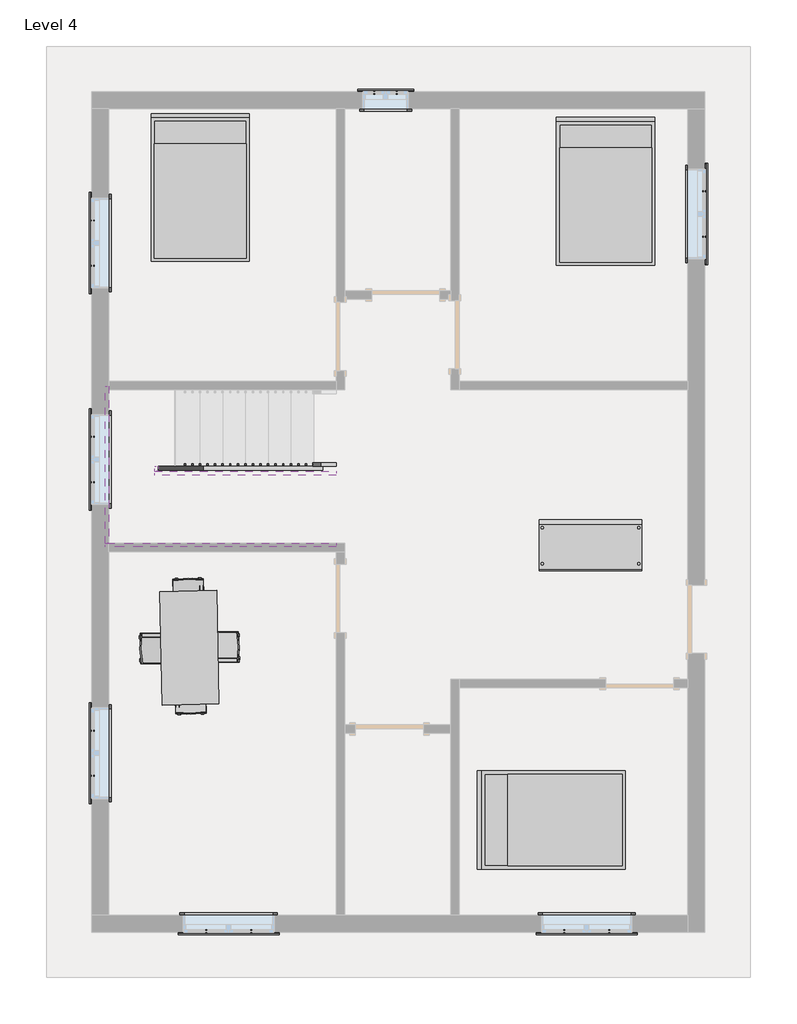
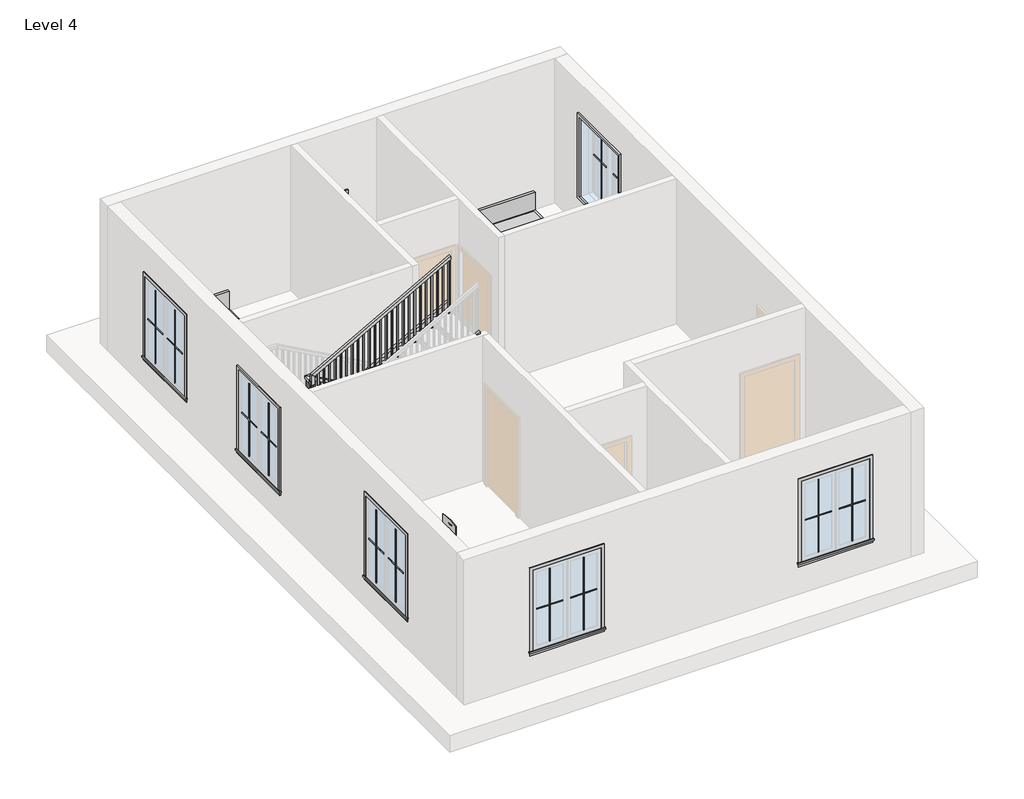
# One storey, part 2 of 2: 29 proxies, 6 members, 4 furniture elements, 1 railing.
"""IFC4 building model written with IfcOpenShell, lengths in millimetres."""

from ifc_helpers import new_model, si_unit, frame, origin, place, context, project, spatial, polyline, outline, extrude, faceted_brep, transform, mapped, element, save
from components import modern_coffee_table_17989_modern_coffee_table_17989_d3a860c8, muntin_pattern_2x2_muntin_pattern_2x2_6dad3731, muntin_pattern_2x2_muntin_pattern_2x2_a30a3345, muntin_pattern_2x2_muntin_pattern_2x2_53152e2c, muntin_pattern_2x2_muntin_pattern_2x2_e8f3e573, trim_window_exterior_flat_with_sill_92b9b949, trim_window_exterior_flat_with_sill_a665a915, trim_window_interior_flat_picture_frame_3bb882cf, trim_window_interior_flat_picture_frame_d485c387, bed_17739_bed_17739_15c61121, dining_table_w_chairs_11374_0cdfc61b

model = new_model("IFC4")

# Units and contexts
model_context = context("Model", 3, world=origin())
ifc_project = project(units=[si_unit("LENGTHUNIT", "METRE", prefix="MILLI")], contexts=[model_context])

# Site, building, storey
site = spatial("IfcSite", under=ifc_project)
building = spatial("IfcBuilding", under=site)
storey = spatial("IfcBuildingStorey", under=building, Name="Level 4", Elevation=9144.0)

# Proxies
placement = place(None, origin())
modern_coffee_table_17989_modern_coffee_table_17989_shape = modern_coffee_table_17989_modern_coffee_table_17989_d3a860c8(model_context)
element("IfcBuildingElementProxy", 1, Name="Modern_Coffee_Table_17989 : Modern_Coffee_Table_17989", ObjectType="Modern_Coffee_Table_17989 : Modern_Coffee_Table_17989", at=placement, inside=storey, context=model_context, shape_type="MappedRepresentation", body=[
    mapped(modern_coffee_table_17989_modern_coffee_table_17989_shape, transform((7937.5, 8234.1992646, 9144.0), x_axis=(1.0, 0.0, 0.0), y_axis=(0.0, 1.0, 0.0), z_axis=(0.0, 0.0, 1.0))),
])
muntin_pattern_2x2_muntin_pattern_2x2_shape = muntin_pattern_2x2_muntin_pattern_2x2_6dad3731(model_context)
element("IfcBuildingElementProxy", 2, Name="Muntin Pattern_2x2 : Muntin Pattern_2x2", ObjectType="Muntin Pattern_2x2 : Muntin Pattern_2x2", at=placement, inside=storey, context=model_context, shape_type="MappedRepresentation", body=[
    mapped(muntin_pattern_2x2_muntin_pattern_2x2_shape, transform((7961.3125, 2701.925, 10128.25), x_axis=(-1.0, 0.0, 0.0), y_axis=(0.0, -1.0, 0.0), z_axis=(0.0, 0.0, 1.0))),
])
element("IfcBuildingElementProxy", 3, Name="Muntin Pattern_2x2 : Muntin Pattern_2x2", ObjectType="Muntin Pattern_2x2 : Muntin Pattern_2x2", at=placement, inside=storey, context=model_context, shape_type="MappedRepresentation", body=[
    mapped(muntin_pattern_2x2_muntin_pattern_2x2_shape, transform((3154.3625, 2701.925, 10128.25), x_axis=(-1.0, 0.0, 0.0), y_axis=(0.0, -1.0, 0.0), z_axis=(0.0, 0.0, 1.0))),
])
element("IfcBuildingElementProxy", 4, Name="Muntin Pattern_2x2 : Muntin Pattern_2x2", ObjectType="Muntin Pattern_2x2 : Muntin Pattern_2x2", at=placement, inside=storey, context=model_context, shape_type="MappedRepresentation", body=[
    mapped(muntin_pattern_2x2_muntin_pattern_2x2_shape, transform((1025.525, 4789.4875, 10128.25), x_axis=(0.0, 1.0, 0.0), y_axis=(-1.0, 0.0, 0.0), z_axis=(0.0, 0.0, 1.0))),
])
element("IfcBuildingElementProxy", 5, Name="Muntin Pattern_2x2 : Muntin Pattern_2x2", ObjectType="Muntin Pattern_2x2 : Muntin Pattern_2x2", at=placement, inside=storey, context=model_context, shape_type="MappedRepresentation", body=[
    mapped(muntin_pattern_2x2_muntin_pattern_2x2_shape, transform((1025.525, 8732.8375, 10128.25), x_axis=(0.0, 1.0, 0.0), y_axis=(-1.0, 0.0, 0.0), z_axis=(0.0, 0.0, 1.0))),
])
element("IfcBuildingElementProxy", 6, Name="Muntin Pattern_2x2 : Muntin Pattern_2x2", ObjectType="Muntin Pattern_2x2 : Muntin Pattern_2x2", at=placement, inside=storey, context=model_context, shape_type="MappedRepresentation", body=[
    mapped(muntin_pattern_2x2_muntin_pattern_2x2_shape, transform((1025.525, 11637.9625, 10128.25), x_axis=(0.0, 1.0, 0.0), y_axis=(-1.0, 0.0, 0.0), z_axis=(0.0, 0.0, 1.0))),
])
element("IfcBuildingElementProxy", 7, Name="Muntin Pattern_2x2 : Muntin Pattern_2x2", ObjectType="Muntin Pattern_2x2 : Muntin Pattern_2x2", at=placement, inside=storey, context=model_context, shape_type="MappedRepresentation", body=[
    mapped(muntin_pattern_2x2_muntin_pattern_2x2_shape, transform((9236.075, 12634.9125, 10128.25), x_axis=(0.0, -1.0, 0.0), y_axis=(1.0, 0.0, 0.0), z_axis=(0.0, 0.0, 1.0))),
])
muntin_pattern_2x2_muntin_pattern_2x2_2_shape = muntin_pattern_2x2_muntin_pattern_2x2_a30a3345(model_context)
element("IfcBuildingElementProxy", 8, Name="Muntin Pattern_2x2 : Muntin Pattern_2x2", ObjectType="Muntin Pattern_2x2 : Muntin Pattern_2x2", at=placement, inside=storey, context=model_context, shape_type="MappedRepresentation", body=[
    mapped(muntin_pattern_2x2_muntin_pattern_2x2_2_shape, transform((7354.8875, 2701.925, 10128.25), x_axis=(1.0, 0.0, 0.0), y_axis=(0.0, 1.0, 0.0), z_axis=(0.0, 0.0, 1.0))),
])
element("IfcBuildingElementProxy", 9, Name="Muntin Pattern_2x2 : Muntin Pattern_2x2", ObjectType="Muntin Pattern_2x2 : Muntin Pattern_2x2", at=placement, inside=storey, context=model_context, shape_type="MappedRepresentation", body=[
    mapped(muntin_pattern_2x2_muntin_pattern_2x2_2_shape, transform((2547.9375, 2701.925, 10128.25), x_axis=(1.0, 0.0, 0.0), y_axis=(0.0, 1.0, 0.0), z_axis=(0.0, 0.0, 1.0))),
])
element("IfcBuildingElementProxy", 10, Name="Muntin Pattern_2x2 : Muntin Pattern_2x2", ObjectType="Muntin Pattern_2x2 : Muntin Pattern_2x2", at=placement, inside=storey, context=model_context, shape_type="MappedRepresentation", body=[
    mapped(muntin_pattern_2x2_muntin_pattern_2x2_2_shape, transform((1025.525, 5395.9125, 10128.25), x_axis=(0.0, -1.0, 0.0), y_axis=(1.0, 0.0, 0.0), z_axis=(0.0, 0.0, 1.0))),
])
element("IfcBuildingElementProxy", 11, Name="Muntin Pattern_2x2 : Muntin Pattern_2x2", ObjectType="Muntin Pattern_2x2 : Muntin Pattern_2x2", at=placement, inside=storey, context=model_context, shape_type="MappedRepresentation", body=[
    mapped(muntin_pattern_2x2_muntin_pattern_2x2_2_shape, transform((1025.525, 9339.2625, 10128.25), x_axis=(0.0, -1.0, 0.0), y_axis=(1.0, 0.0, 0.0), z_axis=(0.0, 0.0, 1.0))),
])
element("IfcBuildingElementProxy", 12, Name="Muntin Pattern_2x2 : Muntin Pattern_2x2", ObjectType="Muntin Pattern_2x2 : Muntin Pattern_2x2", at=placement, inside=storey, context=model_context, shape_type="MappedRepresentation", body=[
    mapped(muntin_pattern_2x2_muntin_pattern_2x2_2_shape, transform((1025.525, 12244.3875, 10128.25), x_axis=(0.0, -1.0, 0.0), y_axis=(1.0, 0.0, 0.0), z_axis=(0.0, 0.0, 1.0))),
])
element("IfcBuildingElementProxy", 13, Name="Muntin Pattern_2x2 : Muntin Pattern_2x2", ObjectType="Muntin Pattern_2x2 : Muntin Pattern_2x2", at=placement, inside=storey, context=model_context, shape_type="MappedRepresentation", body=[
    mapped(muntin_pattern_2x2_muntin_pattern_2x2_2_shape, transform((9236.075, 12028.4875, 10128.25), x_axis=(0.0, 1.0, 0.0), y_axis=(-1.0, 0.0, 0.0), z_axis=(0.0, 0.0, 1.0))),
])
muntin_pattern_2x2_muntin_pattern_2x2_3_shape = muntin_pattern_2x2_muntin_pattern_2x2_53152e2c(model_context)
element("IfcBuildingElementProxy", 14, Name="Muntin Pattern_2x2 : Muntin Pattern_2x2", ObjectType="Muntin Pattern_2x2 : Muntin Pattern_2x2", at=placement, inside=storey, context=model_context, shape_type="MappedRepresentation", body=[
    mapped(muntin_pattern_2x2_muntin_pattern_2x2_3_shape, transform((4808.5375, 13960.475, 10128.25), x_axis=(1.0, 0.0, 0.0), y_axis=(0.0, 1.0, 0.0), z_axis=(0.0, 0.0, 1.0))),
])
muntin_pattern_2x2_muntin_pattern_2x2_4_shape = muntin_pattern_2x2_muntin_pattern_2x2_e8f3e573(model_context)
element("IfcBuildingElementProxy", 15, Name="Muntin Pattern_2x2 : Muntin Pattern_2x2", ObjectType="Muntin Pattern_2x2 : Muntin Pattern_2x2", at=placement, inside=storey, context=model_context, shape_type="MappedRepresentation", body=[
    mapped(muntin_pattern_2x2_muntin_pattern_2x2_4_shape, transform((5110.1625, 13960.475, 10128.25), x_axis=(-1.0, 0.0, 0.0), y_axis=(0.0, -1.0, 0.0), z_axis=(0.0, 0.0, 1.0))),
])
trim_window_exterior_flat_with_sill_shape = trim_window_exterior_flat_with_sill_92b9b949(model_context)
element("IfcBuildingElementProxy", 16, Name="Trim-Window-Exterior-Flat : with Sill", ObjectType="Trim-Window-Exterior-Flat : with Sill", at=placement, inside=storey, context=model_context, shape_type="MappedRepresentation", body=[
    mapped(trim_window_exterior_flat_with_sill_shape, transform((7658.1, 2692.4, 11582.4), x_axis=(1.0, 0.0, 0.0), y_axis=(0.0, 0.0, 1.0), z_axis=(0.0, -1.0, 0.0))),
])
element("IfcBuildingElementProxy", 17, Name="Trim-Window-Exterior-Flat : with Sill", ObjectType="Trim-Window-Exterior-Flat : with Sill", at=placement, inside=storey, context=model_context, shape_type="MappedRepresentation", body=[
    mapped(trim_window_exterior_flat_with_sill_shape, transform((2851.15, 2692.4, 11582.4), x_axis=(1.0, 0.0, 0.0), y_axis=(0.0, 0.0, 1.0), z_axis=(0.0, -1.0, 0.0))),
])
element("IfcBuildingElementProxy", 18, Name="Trim-Window-Exterior-Flat : with Sill", ObjectType="Trim-Window-Exterior-Flat : with Sill", at=placement, inside=storey, context=model_context, shape_type="MappedRepresentation", body=[
    mapped(trim_window_exterior_flat_with_sill_shape, transform((1016.0, 5092.7, 11582.4), x_axis=(0.0, -1.0, 0.0), y_axis=(0.0, 0.0, 1.0), z_axis=(-1.0, 0.0, 0.0))),
])
element("IfcBuildingElementProxy", 19, Name="Trim-Window-Exterior-Flat : with Sill", ObjectType="Trim-Window-Exterior-Flat : with Sill", at=placement, inside=storey, context=model_context, shape_type="MappedRepresentation", body=[
    mapped(trim_window_exterior_flat_with_sill_shape, transform((1016.0, 9036.05, 11582.4), x_axis=(0.0, -1.0, 0.0), y_axis=(0.0, 0.0, 1.0), z_axis=(-1.0, 0.0, 0.0))),
])
element("IfcBuildingElementProxy", 20, Name="Trim-Window-Exterior-Flat : with Sill", ObjectType="Trim-Window-Exterior-Flat : with Sill", at=placement, inside=storey, context=model_context, shape_type="MappedRepresentation", body=[
    mapped(trim_window_exterior_flat_with_sill_shape, transform((1016.0, 11941.175, 11582.4), x_axis=(0.0, -1.0, 0.0), y_axis=(0.0, 0.0, 1.0), z_axis=(-1.0, 0.0, 0.0))),
])
element("IfcBuildingElementProxy", 21, Name="Trim-Window-Exterior-Flat : with Sill", ObjectType="Trim-Window-Exterior-Flat : with Sill", at=placement, inside=storey, context=model_context, shape_type="MappedRepresentation", body=[
    mapped(trim_window_exterior_flat_with_sill_shape, transform((9245.6, 12331.7, 11582.4), x_axis=(0.0, 1.0, 0.0), y_axis=(0.0, 0.0, 1.0), z_axis=(1.0, 0.0, 0.0))),
])
trim_window_exterior_flat_with_sill_2_shape = trim_window_exterior_flat_with_sill_a665a915(model_context)
element("IfcBuildingElementProxy", 22, Name="Trim-Window-Exterior-Flat : with Sill", ObjectType="Trim-Window-Exterior-Flat : with Sill", at=placement, inside=storey, context=model_context, shape_type="MappedRepresentation", body=[
    mapped(trim_window_exterior_flat_with_sill_2_shape, transform((4959.35, 13970.0, 10972.8), x_axis=(-1.0, 0.0, 0.0), y_axis=(0.0, 0.0, 1.0), z_axis=(0.0, 1.0, 0.0))),
])
trim_window_interior_flat_picture_frame_shape = trim_window_interior_flat_picture_frame_3bb882cf(model_context)
element("IfcBuildingElementProxy", 23, Name="Trim-Window-Interior-Flat : Picture Frame", ObjectType="Trim-Window-Interior-Flat : Picture Frame", at=placement, inside=storey, context=model_context, shape_type="MappedRepresentation", body=[
    mapped(trim_window_interior_flat_picture_frame_shape, transform((7658.1, 2921.0, 11582.4), x_axis=(-1.0, 0.0, 0.0), y_axis=(0.0, 0.0, 1.0), z_axis=(0.0, 1.0, 0.0))),
])
element("IfcBuildingElementProxy", 24, Name="Trim-Window-Interior-Flat : Picture Frame", ObjectType="Trim-Window-Interior-Flat : Picture Frame", at=placement, inside=storey, context=model_context, shape_type="MappedRepresentation", body=[
    mapped(trim_window_interior_flat_picture_frame_shape, transform((2851.15, 2921.0, 11582.4), x_axis=(-1.0, 0.0, 0.0), y_axis=(0.0, 0.0, 1.0), z_axis=(0.0, 1.0, 0.0))),
])
element("IfcBuildingElementProxy", 25, Name="Trim-Window-Interior-Flat : Picture Frame", ObjectType="Trim-Window-Interior-Flat : Picture Frame", at=placement, inside=storey, context=model_context, shape_type="MappedRepresentation", body=[
    mapped(trim_window_interior_flat_picture_frame_shape, transform((1244.6, 5092.7, 11582.4), x_axis=(0.0, 1.0, 0.0), y_axis=(0.0, 0.0, 1.0), z_axis=(1.0, 0.0, 0.0))),
])
element("IfcBuildingElementProxy", 26, Name="Trim-Window-Interior-Flat : Picture Frame", ObjectType="Trim-Window-Interior-Flat : Picture Frame", at=placement, inside=storey, context=model_context, shape_type="MappedRepresentation", body=[
    mapped(trim_window_interior_flat_picture_frame_shape, transform((1244.6, 9036.05, 11582.4), x_axis=(0.0, 1.0, 0.0), y_axis=(0.0, 0.0, 1.0), z_axis=(1.0, 0.0, 0.0))),
])
element("IfcBuildingElementProxy", 27, Name="Trim-Window-Interior-Flat : Picture Frame", ObjectType="Trim-Window-Interior-Flat : Picture Frame", at=placement, inside=storey, context=model_context, shape_type="MappedRepresentation", body=[
    mapped(trim_window_interior_flat_picture_frame_shape, transform((1244.6, 11941.175, 11582.4), x_axis=(0.0, 1.0, 0.0), y_axis=(0.0, 0.0, 1.0), z_axis=(1.0, 0.0, 0.0))),
])
element("IfcBuildingElementProxy", 28, Name="Trim-Window-Interior-Flat : Picture Frame", ObjectType="Trim-Window-Interior-Flat : Picture Frame", at=placement, inside=storey, context=model_context, shape_type="MappedRepresentation", body=[
    mapped(trim_window_interior_flat_picture_frame_shape, transform((9017.0, 12331.7, 11582.4), x_axis=(0.0, -1.0, 0.0), y_axis=(0.0, 0.0, 1.0), z_axis=(-1.0, 0.0, 0.0))),
])
trim_window_interior_flat_picture_frame_2_shape = trim_window_interior_flat_picture_frame_d485c387(model_context)
element("IfcBuildingElementProxy", 29, Name="Trim-Window-Interior-Flat : Picture Frame", ObjectType="Trim-Window-Interior-Flat : Picture Frame", at=placement, inside=storey, context=model_context, shape_type="MappedRepresentation", body=[
    mapped(trim_window_interior_flat_picture_frame_2_shape, transform((4959.35, 13741.4, 10972.8), x_axis=(1.0, 0.0, 0.0), y_axis=(0.0, 0.0, 1.0), z_axis=(0.0, -1.0, 0.0))),
])

# Furniture
bed_17739_bed_17739_shape = bed_17739_bed_17739_15c61121(model_context)
element("IfcFurniture", 30, ObjectType="Bed_17739 : Bed_17739", at=placement, inside=storey, context=model_context, shape_type="MappedRepresentation", body=[
    mapped(bed_17739_bed_17739_shape, transform((2470.15, 12661.9, 9144.0), x_axis=(1.0, 0.0, 0.0), y_axis=(0.0, 1.0, 0.0), z_axis=(0.0, 0.0, 1.0))),
])
element("IfcFurniture", 31, ObjectType="Bed_17739 : Bed_17739", at=placement, inside=storey, context=model_context, shape_type="MappedRepresentation", body=[
    mapped(bed_17739_bed_17739_shape, transform((7912.1, 12611.1, 9144.0), x_axis=(1.0, 0.0, 0.0), y_axis=(0.0, 1.0, 0.0), z_axis=(0.0, 0.0, 1.0))),
])
element("IfcFurniture", 32, ObjectType="Bed_17739 : Bed_17739", at=placement, inside=storey, context=model_context, shape_type="MappedRepresentation", body=[
    mapped(bed_17739_bed_17739_shape, transform((7207.25, 4197.35, 9144.0), x_axis=(0.0, 1.0, 0.0), y_axis=(-1.0, 0.0, 0.0), z_axis=(0.0, 0.0, 1.0))),
])
dining_table_w_chairs_11374_shape = dining_table_w_chairs_11374_0cdfc61b(model_context)
element("IfcFurniture", 33, ObjectType="Dining_Table_w_Chairs_11374", at=placement, inside=storey, context=model_context, shape_type="MappedRepresentation", body=[
    mapped(dining_table_w_chairs_11374_shape, transform((2420.6366388, 6492.5326572, 9144.0), x_axis=(-0.019560245774115807, 0.9998086800909743, 0.0), y_axis=(-0.9998086800909743, -0.019560245774115807, 0.0), z_axis=(0.0, 0.0, 1.0))),
])

# Members
element("IfcMember", 34, ObjectType="Stringer - 2\" Width", at=placement, inside=storey, context=model_context, shape_type="SweptSolid", body=[
    extrude(outline(polyline([(9144.0, 4295.1355783), (9351.5983948, 4295.1355783), (10678.0428392, 1907.5355783), (10329.3641651, 1907.5355783), (9144.0, 4041.1910755), (9144.0, 4295.1355783)])), frame((0.0, 8893.8068332, 0.0), z_axis=(0.0, 1.0, 0.0), x_axis=(0.0, 0.0, 1.0)), (0.0, 0.0, 1.0), 50.8),
])
element("IfcMember", 35, ObjectType="Stringer - 2\" Width", at=placement, inside=storey, context=model_context, shape_type="SweptSolid", body=[
    extrude(outline(polyline([(1856.7355783, 8944.6068332), (1907.5355783, 8944.6068332), (1907.5355783, 8877.3), (1856.7355783, 8877.3), (1856.7355783, 8944.6068332)])), frame((0.0, 0.0, 10439.4), z_axis=(0.0, 0.0, 1.0), x_axis=(1.0, 0.0, 0.0)), (0.0, 0.0, 1.0), 304.8),
])
element("IfcMember", 36, ObjectType="Stringer - 2\" Width", at=placement, inside=storey, context=model_context, shape_type="SweptSolid", body=[
    extrude(outline(polyline([(10875.5983948, 1856.7355783), (10526.9197207, 1856.7355783), (11881.5863873, 4295.1355783), (12230.2650614, 4295.1355783), (10875.5983948, 1856.7355783)])), frame((0.0, 8826.5, 0.0), z_axis=(0.0, 1.0, 0.0), x_axis=(0.0, 0.0, 1.0)), (0.0, 0.0, 1.0), 50.8),
])
element("IfcMember", 37, ObjectType="Stringer - 2\" Width", at=placement, inside=storey, context=model_context, shape_type="SweptSolid", body=[
    extrude(outline(polyline([(9144.0, 4295.1355783), (9351.5983948, 4295.1355783), (10744.2, 1788.4526889), (10744.2, 1244.6), (10697.6617086, 1244.6), (9144.0, 4041.1910755), (9144.0, 4295.1355783)])), frame((0.0, 9969.5, 0.0), z_axis=(0.0, 1.0, 0.0), x_axis=(0.0, 0.0, 1.0)), (0.0, 0.0, 1.0), 50.8),
])
element("IfcMember", 38, ObjectType="Stringer - 2\" Width", at=placement, inside=storey, context=model_context, shape_type="SweptSolid", body=[
    extrude(outline(polyline([(1193.8, 10020.3), (1244.6, 10020.3), (1244.6, 7912.1), (1193.8, 7912.1), (1193.8, 10020.3)])), frame((0.0, 0.0, 10439.4), z_axis=(0.0, 0.0, 1.0), x_axis=(1.0, 0.0, 0.0)), (0.0, 0.0, 1.0), 304.8),
])
element("IfcMember", 39, ObjectType="Stringer - 2\" Width", at=placement, inside=storey, context=model_context, shape_type="SweptSolid", body=[
    extrude(outline(polyline([(10507.3008513, 1193.8), (10439.4, 1193.8), (10439.4, 1699.2000811), (11881.5863873, 4295.1355783), (12230.2650614, 4295.1355783), (10507.3008513, 1193.8)])), frame((0.0, 7861.3, 0.0), z_axis=(0.0, 1.0, 0.0), x_axis=(0.0, 0.0, 1.0)), (0.0, 0.0, 1.0), 50.8),
])

# Railing
element("IfcRailing", 40, ObjectType="Handrail - Rectangular", at=placement, inside=storey, context=model_context, shape_type="SolidModel", body=[
    faceted_brep([(4295.1355783, 8944.6068332, 10227.7333333), (4295.1355783, 8944.6068332, 10169.620221), (4295.1355783, 8995.4068332, 10169.620221), (4295.1355783, 8995.4068332, 10227.7333333), (1932.9355783, 8944.6068332, 11540.0666667), (1882.1355783, 8944.6068332, 11510.1757765), (1882.1355783, 8995.4068332, 11510.1757765), (1932.9355783, 8995.4068332, 11540.0666667), (1932.9355783, 8944.6068332, 11582.4), (1882.1355783, 8944.6068332, 11531.6), (1882.1355783, 8995.4068332, 11531.6), (1932.9355783, 8995.4068332, 11582.4), (1856.7355783, 8944.6068332, 11582.4), (1856.7355783, 8944.6068332, 11531.6), (1805.9355783, 8995.4068332, 11531.6), (1805.9355783, 8995.4068332, 11582.4), (1856.7355783, 8868.4068332, 11582.4), (1856.7355783, 8868.4068332, 11531.6), (1805.9355783, 8868.4068332, 11531.6), (1805.9355783, 8868.4068332, 11582.4), (1856.7355783, 8826.5, 11582.4), (1805.9355783, 8826.5, 11582.4), (1805.9355783, 8775.7, 11531.6), (1856.7355783, 8775.7, 11531.6)], [[[0, 1, 2, 3]], [[1, 0, 4, 5]], [[2, 1, 5, 6]], [[3, 2, 6, 7]], [[0, 3, 7, 4]], [[5, 4, 8, 9]], [[6, 5, 9, 10]], [[7, 6, 10, 11]], [[4, 7, 11, 8]], [[9, 8, 12, 13]], [[10, 9, 13, 14]], [[11, 10, 14, 15]], [[8, 11, 15, 12]], [[13, 12, 16, 17]], [[14, 13, 17, 18]], [[15, 14, 18, 19]], [[12, 15, 19, 16]], [[20, 21, 22, 23]], [[17, 16, 20, 23]], [[18, 17, 23, 22]], [[19, 18, 22, 21]], [[16, 19, 21, 20]]]),
    faceted_brep([(1856.7355783, 8826.5, 11582.4), (1856.7355783, 8775.7, 11531.6), (1805.9355783, 8775.7, 11531.6), (1805.9355783, 8826.5, 11582.4), (1856.7355783, 8826.5, 11693.620221), (1805.9355783, 8826.5, 11723.5111111), (1805.9355783, 8775.7, 11723.5111111), (1856.7355783, 8775.7, 11693.620221)], [[[0, 1, 2, 3]], [[4, 5, 6, 7]], [[1, 0, 4, 7]], [[2, 1, 7, 6]], [[3, 2, 6, 5]], [[0, 3, 5, 4]]]),
    faceted_brep([(1805.9355783, 8826.5, 11723.5111111), (1856.7355783, 8826.5, 11693.620221), (1856.7355783, 8775.7, 11693.620221), (1805.9355783, 8775.7, 11723.5111111), (4295.1355783, 8826.5, 13106.4), (4295.1355783, 8775.7, 13106.4), (4295.1355783, 8775.7, 13048.2868876), (4295.1355783, 8826.5, 13048.2868876)], [[[0, 1, 2, 3]], [[4, 5, 6, 7]], [[1, 0, 4, 7]], [[2, 1, 7, 6]], [[3, 2, 6, 5]], [[0, 3, 5, 4]]]),
    extrude(outline(polyline([(13028.8841099, 4260.2105783), (12022.6666667, 4260.2105783), (12022.6666667, 4279.2605783), (13039.4674432, 4279.2605783), (13028.8841099, 4260.2105783)])), frame((0.0, 8791.575, 0.0), z_axis=(0.0, 1.0, 0.0), x_axis=(0.0, 0.0, 1.0)), (0.0, 0.0, 1.0), 19.05),
    extrude(outline(polyline([(12972.4396654, 4158.6105783), (12022.6666667, 4158.6105783), (12022.6666667, 4177.6605783), (12983.0229988, 4177.6605783), (12972.4396654, 4158.6105783)])), frame((0.0, 8791.575, 0.0), z_axis=(0.0, 1.0, 0.0), x_axis=(0.0, 0.0, 1.0)), (0.0, 0.0, 1.0), 19.05),
    extrude(outline(polyline([(12915.995221, 4057.0105783), (12022.6666667, 4057.0105783), (12022.6666667, 4076.0605783), (12926.5785543, 4076.0605783), (12915.995221, 4057.0105783)])), frame((0.0, 8791.575, 0.0), z_axis=(0.0, 1.0, 0.0), x_axis=(0.0, 0.0, 1.0)), (0.0, 0.0, 1.0), 19.05),
    extrude(outline(polyline([(12859.5507765, 3955.4105783), (11853.3333333, 3955.4105783), (11853.3333333, 3974.4605783), (12870.1341099, 3974.4605783), (12859.5507765, 3955.4105783)])), frame((0.0, 8791.575, 0.0), z_axis=(0.0, 1.0, 0.0), x_axis=(0.0, 0.0, 1.0)), (0.0, 0.0, 1.0), 19.05),
    extrude(outline(polyline([(12803.1063321, 3853.8105783), (11853.3333333, 3853.8105783), (11853.3333333, 3872.8605783), (12813.6896654, 3872.8605783), (12803.1063321, 3853.8105783)])), frame((0.0, 8791.575, 0.0), z_axis=(0.0, 1.0, 0.0), x_axis=(0.0, 0.0, 1.0)), (0.0, 0.0, 1.0), 19.05),
    extrude(outline(polyline([(12746.6618876, 3752.2105783), (11853.3333333, 3752.2105783), (11853.3333333, 3771.2605783), (12757.245221, 3771.2605783), (12746.6618876, 3752.2105783)])), frame((0.0, 8791.575, 0.0), z_axis=(0.0, 1.0, 0.0), x_axis=(0.0, 0.0, 1.0)), (0.0, 0.0, 1.0), 19.05),
    extrude(outline(polyline([(12690.2174432, 3650.6105783), (11684.0, 3650.6105783), (11684.0, 3669.6605783), (12700.8007765, 3669.6605783), (12690.2174432, 3650.6105783)])), frame((0.0, 8791.575, 0.0), z_axis=(0.0, 1.0, 0.0), x_axis=(0.0, 0.0, 1.0)), (0.0, 0.0, 1.0), 19.05),
    extrude(outline(polyline([(12633.7729988, 3549.0105783), (11684.0, 3549.0105783), (11684.0, 3568.0605783), (12644.3563321, 3568.0605783), (12633.7729988, 3549.0105783)])), frame((0.0, 8791.575, 0.0), z_axis=(0.0, 1.0, 0.0), x_axis=(0.0, 0.0, 1.0)), (0.0, 0.0, 1.0), 19.05),
    extrude(outline(polyline([(12577.3285543, 3447.4105783), (11684.0, 3447.4105783), (11684.0, 3466.4605783), (12587.9118876, 3466.4605783), (12577.3285543, 3447.4105783)])), frame((0.0, 8791.575, 0.0), z_axis=(0.0, 1.0, 0.0), x_axis=(0.0, 0.0, 1.0)), (0.0, 0.0, 1.0), 19.05),
    extrude(outline(polyline([(12520.8841099, 3345.8105783), (11514.6666667, 3345.8105783), (11514.6666667, 3364.8605783), (12531.4674432, 3364.8605783), (12520.8841099, 3345.8105783)])), frame((0.0, 8791.575, 0.0), z_axis=(0.0, 1.0, 0.0), x_axis=(0.0, 0.0, 1.0)), (0.0, 0.0, 1.0), 19.05),
    extrude(outline(polyline([(12464.4396654, 3244.2105783), (11514.6666667, 3244.2105783), (11514.6666667, 3263.2605783), (12475.0229988, 3263.2605783), (12464.4396654, 3244.2105783)])), frame((0.0, 8791.575, 0.0), z_axis=(0.0, 1.0, 0.0), x_axis=(0.0, 0.0, 1.0)), (0.0, 0.0, 1.0), 19.05),
    extrude(outline(polyline([(12407.995221, 3142.6105783), (11514.6666667, 3142.6105783), (11514.6666667, 3161.6605783), (12418.5785543, 3161.6605783), (12407.995221, 3142.6105783)])), frame((0.0, 8791.575, 0.0), z_axis=(0.0, 1.0, 0.0), x_axis=(0.0, 0.0, 1.0)), (0.0, 0.0, 1.0), 19.05),
    extrude(outline(polyline([(12351.5507765, 3041.0105783), (11345.3333333, 3041.0105783), (11345.3333333, 3060.0605783), (12362.1341099, 3060.0605783), (12351.5507765, 3041.0105783)])), frame((0.0, 8791.575, 0.0), z_axis=(0.0, 1.0, 0.0), x_axis=(0.0, 0.0, 1.0)), (0.0, 0.0, 1.0), 19.05),
    extrude(outline(polyline([(12295.1063321, 2939.4105783), (11345.3333333, 2939.4105783), (11345.3333333, 2958.4605783), (12305.6896654, 2958.4605783), (12295.1063321, 2939.4105783)])), frame((0.0, 8791.575, 0.0), z_axis=(0.0, 1.0, 0.0), x_axis=(0.0, 0.0, 1.0)), (0.0, 0.0, 1.0), 19.05),
    extrude(outline(polyline([(12238.6618876, 2837.8105783), (11345.3333333, 2837.8105783), (11345.3333333, 2856.8605783), (12249.245221, 2856.8605783), (12238.6618876, 2837.8105783)])), frame((0.0, 8791.575, 0.0), z_axis=(0.0, 1.0, 0.0), x_axis=(0.0, 0.0, 1.0)), (0.0, 0.0, 1.0), 19.05),
    extrude(outline(polyline([(12182.2174432, 2736.2105783), (11176.0, 2736.2105783), (11176.0, 2755.2605783), (12192.8007765, 2755.2605783), (12182.2174432, 2736.2105783)])), frame((0.0, 8791.575, 0.0), z_axis=(0.0, 1.0, 0.0), x_axis=(0.0, 0.0, 1.0)), (0.0, 0.0, 1.0), 19.05),
    extrude(outline(polyline([(12125.7729988, 2634.6105783), (11176.0, 2634.6105783), (11176.0, 2653.6605783), (12136.3563321, 2653.6605783), (12125.7729988, 2634.6105783)])), frame((0.0, 8791.575, 0.0), z_axis=(0.0, 1.0, 0.0), x_axis=(0.0, 0.0, 1.0)), (0.0, 0.0, 1.0), 19.05),
    extrude(outline(polyline([(12069.3285543, 2533.0105783), (11176.0, 2533.0105783), (11176.0, 2552.0605783), (12079.9118876, 2552.0605783), (12069.3285543, 2533.0105783)])), frame((0.0, 8791.575, 0.0), z_axis=(0.0, 1.0, 0.0), x_axis=(0.0, 0.0, 1.0)), (0.0, 0.0, 1.0), 19.05),
    extrude(outline(polyline([(12012.8841099, 2431.4105783), (11006.6666667, 2431.4105783), (11006.6666667, 2450.4605783), (12023.4674432, 2450.4605783), (12012.8841099, 2431.4105783)])), frame((0.0, 8791.575, 0.0), z_axis=(0.0, 1.0, 0.0), x_axis=(0.0, 0.0, 1.0)), (0.0, 0.0, 1.0), 19.05),
    extrude(outline(polyline([(11956.4396654, 2329.8105783), (11006.6666667, 2329.8105783), (11006.6666667, 2348.8605783), (11967.0229988, 2348.8605783), (11956.4396654, 2329.8105783)])), frame((0.0, 8791.575, 0.0), z_axis=(0.0, 1.0, 0.0), x_axis=(0.0, 0.0, 1.0)), (0.0, 0.0, 1.0), 19.05),
    extrude(outline(polyline([(11899.995221, 2228.2105783), (11006.6666667, 2228.2105783), (11006.6666667, 2247.2605783), (11910.5785543, 2247.2605783), (11899.995221, 2228.2105783)])), frame((0.0, 8791.575, 0.0), z_axis=(0.0, 1.0, 0.0), x_axis=(0.0, 0.0, 1.0)), (0.0, 0.0, 1.0), 19.05),
    extrude(outline(polyline([(11843.5507765, 2126.6105783), (10837.3333333, 2126.6105783), (10837.3333333, 2145.6605783), (11854.1341099, 2145.6605783), (11843.5507765, 2126.6105783)])), frame((0.0, 8791.575, 0.0), z_axis=(0.0, 1.0, 0.0), x_axis=(0.0, 0.0, 1.0)), (0.0, 0.0, 1.0), 19.05),
    extrude(outline(polyline([(11787.1063321, 2025.0105783), (10837.3333333, 2025.0105783), (10837.3333333, 2044.0605783), (11797.6896654, 2044.0605783), (11787.1063321, 2025.0105783)])), frame((0.0, 8791.575, 0.0), z_axis=(0.0, 1.0, 0.0), x_axis=(0.0, 0.0, 1.0)), (0.0, 0.0, 1.0), 19.05),
    extrude(outline(polyline([(11730.6618876, 1923.4105783), (10837.3333333, 1923.4105783), (10837.3333333, 1942.4605783), (11741.245221, 1942.4605783), (11730.6618876, 1923.4105783)])), frame((0.0, 8791.575, 0.0), z_axis=(0.0, 1.0, 0.0), x_axis=(0.0, 0.0, 1.0)), (0.0, 0.0, 1.0), 19.05),
    extrude(outline(polyline([(1840.8605783, 8877.9318332), (1840.8605783, 8858.8818332), (1821.8105783, 8858.8818332), (1821.8105783, 8877.9318332), (1840.8605783, 8877.9318332)])), frame((0.0, 0.0, 10668.0), z_axis=(0.0, 0.0, 1.0), x_axis=(1.0, 0.0, 0.0)), (0.0, 0.0, 1.0), 863.6),
    extrude(outline(polyline([(1866.2605783, 8960.4818332), (1847.2105783, 8960.4818332), (1847.2105783, 8979.5318332), (1866.2605783, 8979.5318332), (1866.2605783, 8960.4818332)])), frame((0.0, 0.0, 10668.0), z_axis=(0.0, 0.0, 1.0), x_axis=(1.0, 0.0, 0.0)), (0.0, 0.0, 1.0), 863.6),
    extrude(outline(polyline([(11473.1341099, 1948.8105783), (10498.6666667, 1948.8105783), (10498.6666667, 1967.8605783), (11462.5507765, 1967.8605783), (11473.1341099, 1948.8105783)])), frame((0.0, 8960.4818332, 0.0), z_axis=(0.0, 1.0, 0.0), x_axis=(0.0, 0.0, 1.0)), (0.0, 0.0, 1.0), 19.05),
    extrude(outline(polyline([(11416.6896654, 2050.4105783), (10498.6666667, 2050.4105783), (10498.6666667, 2069.4605783), (11406.1063321, 2069.4605783), (11416.6896654, 2050.4105783)])), frame((0.0, 8960.4818332, 0.0), z_axis=(0.0, 1.0, 0.0), x_axis=(0.0, 0.0, 1.0)), (0.0, 0.0, 1.0), 19.05),
    extrude(outline(polyline([(11360.245221, 2152.0105783), (10498.6666667, 2152.0105783), (10498.6666667, 2171.0605783), (11349.6618876, 2171.0605783), (11360.245221, 2152.0105783)])), frame((0.0, 8960.4818332, 0.0), z_axis=(0.0, 1.0, 0.0), x_axis=(0.0, 0.0, 1.0)), (0.0, 0.0, 1.0), 19.05),
    extrude(outline(polyline([(11303.8007765, 2253.6105783), (10329.3333333, 2253.6105783), (10329.3333333, 2272.6605783), (11293.2174432, 2272.6605783), (11303.8007765, 2253.6105783)])), frame((0.0, 8960.4818332, 0.0), z_axis=(0.0, 1.0, 0.0), x_axis=(0.0, 0.0, 1.0)), (0.0, 0.0, 1.0), 19.05),
    extrude(outline(polyline([(11247.3563321, 2355.2105783), (10329.3333333, 2355.2105783), (10329.3333333, 2374.2605783), (11236.7729988, 2374.2605783), (11247.3563321, 2355.2105783)])), frame((0.0, 8960.4818332, 0.0), z_axis=(0.0, 1.0, 0.0), x_axis=(0.0, 0.0, 1.0)), (0.0, 0.0, 1.0), 19.05),
    extrude(outline(polyline([(11190.9118876, 2456.8105783), (10329.3333333, 2456.8105783), (10329.3333333, 2475.8605783), (11180.3285543, 2475.8605783), (11190.9118876, 2456.8105783)])), frame((0.0, 8960.4818332, 0.0), z_axis=(0.0, 1.0, 0.0), x_axis=(0.0, 0.0, 1.0)), (0.0, 0.0, 1.0), 19.05),
    extrude(outline(polyline([(11134.4674432, 2558.4105783), (10160.0, 2558.4105783), (10160.0, 2577.4605783), (11123.8841099, 2577.4605783), (11134.4674432, 2558.4105783)])), frame((0.0, 8960.4818332, 0.0), z_axis=(0.0, 1.0, 0.0), x_axis=(0.0, 0.0, 1.0)), (0.0, 0.0, 1.0), 19.05),
    extrude(outline(polyline([(11078.0229988, 2660.0105783), (10160.0, 2660.0105783), (10160.0, 2679.0605783), (11067.4396654, 2679.0605783), (11078.0229988, 2660.0105783)])), frame((0.0, 8960.4818332, 0.0), z_axis=(0.0, 1.0, 0.0), x_axis=(0.0, 0.0, 1.0)), (0.0, 0.0, 1.0), 19.05),
    extrude(outline(polyline([(11021.5785543, 2761.6105783), (10160.0, 2761.6105783), (10160.0, 2780.6605783), (11010.995221, 2780.6605783), (11021.5785543, 2761.6105783)])), frame((0.0, 8960.4818332, 0.0), z_axis=(0.0, 1.0, 0.0), x_axis=(0.0, 0.0, 1.0)), (0.0, 0.0, 1.0), 19.05),
    extrude(outline(polyline([(10965.1341099, 2863.2105783), (9990.6666667, 2863.2105783), (9990.6666667, 2882.2605783), (10954.5507765, 2882.2605783), (10965.1341099, 2863.2105783)])), frame((0.0, 8960.4818332, 0.0), z_axis=(0.0, 1.0, 0.0), x_axis=(0.0, 0.0, 1.0)), (0.0, 0.0, 1.0), 19.05),
    extrude(outline(polyline([(10908.6896654, 2964.8105783), (9990.6666667, 2964.8105783), (9990.6666667, 2983.8605783), (10898.1063321, 2983.8605783), (10908.6896654, 2964.8105783)])), frame((0.0, 8960.4818332, 0.0), z_axis=(0.0, 1.0, 0.0), x_axis=(0.0, 0.0, 1.0)), (0.0, 0.0, 1.0), 19.05),
    extrude(outline(polyline([(10852.245221, 3066.4105783), (9990.6666667, 3066.4105783), (9990.6666667, 3085.4605783), (10841.6618876, 3085.4605783), (10852.245221, 3066.4105783)])), frame((0.0, 8960.4818332, 0.0), z_axis=(0.0, 1.0, 0.0), x_axis=(0.0, 0.0, 1.0)), (0.0, 0.0, 1.0), 19.05),
    extrude(outline(polyline([(10795.8007765, 3168.0105783), (9821.3333333, 3168.0105783), (9821.3333333, 3187.0605783), (10785.2174432, 3187.0605783), (10795.8007765, 3168.0105783)])), frame((0.0, 8960.4818332, 0.0), z_axis=(0.0, 1.0, 0.0), x_axis=(0.0, 0.0, 1.0)), (0.0, 0.0, 1.0), 19.05),
    extrude(outline(polyline([(10739.3563321, 3269.6105783), (9821.3333333, 3269.6105783), (9821.3333333, 3288.6605783), (10728.7729988, 3288.6605783), (10739.3563321, 3269.6105783)])), frame((0.0, 8960.4818332, 0.0), z_axis=(0.0, 1.0, 0.0), x_axis=(0.0, 0.0, 1.0)), (0.0, 0.0, 1.0), 19.05),
    extrude(outline(polyline([(10682.9118876, 3371.2105783), (9821.3333333, 3371.2105783), (9821.3333333, 3390.2605783), (10672.3285543, 3390.2605783), (10682.9118876, 3371.2105783)])), frame((0.0, 8960.4818332, 0.0), z_axis=(0.0, 1.0, 0.0), x_axis=(0.0, 0.0, 1.0)), (0.0, 0.0, 1.0), 19.05),
    extrude(outline(polyline([(10626.4674432, 3472.8105783), (9652.0, 3472.8105783), (9652.0, 3491.8605783), (10615.8841099, 3491.8605783), (10626.4674432, 3472.8105783)])), frame((0.0, 8960.4818332, 0.0), z_axis=(0.0, 1.0, 0.0), x_axis=(0.0, 0.0, 1.0)), (0.0, 0.0, 1.0), 19.05),
    extrude(outline(polyline([(10570.0229988, 3574.4105783), (9652.0, 3574.4105783), (9652.0, 3593.4605783), (10559.4396654, 3593.4605783), (10570.0229988, 3574.4105783)])), frame((0.0, 8960.4818332, 0.0), z_axis=(0.0, 1.0, 0.0), x_axis=(0.0, 0.0, 1.0)), (0.0, 0.0, 1.0), 19.05),
    extrude(outline(polyline([(10513.5785543, 3676.0105783), (9652.0, 3676.0105783), (9652.0, 3695.0605783), (10502.995221, 3695.0605783), (10513.5785543, 3676.0105783)])), frame((0.0, 8960.4818332, 0.0), z_axis=(0.0, 1.0, 0.0), x_axis=(0.0, 0.0, 1.0)), (0.0, 0.0, 1.0), 19.05),
    extrude(outline(polyline([(10457.1341099, 3777.6105783), (9482.6666667, 3777.6105783), (9482.6666667, 3796.6605783), (10446.5507765, 3796.6605783), (10457.1341099, 3777.6105783)])), frame((0.0, 8960.4818332, 0.0), z_axis=(0.0, 1.0, 0.0), x_axis=(0.0, 0.0, 1.0)), (0.0, 0.0, 1.0), 19.05),
    extrude(outline(polyline([(10400.6896654, 3879.2105783), (9482.6666667, 3879.2105783), (9482.6666667, 3898.2605783), (10390.1063321, 3898.2605783), (10400.6896654, 3879.2105783)])), frame((0.0, 8960.4818332, 0.0), z_axis=(0.0, 1.0, 0.0), x_axis=(0.0, 0.0, 1.0)), (0.0, 0.0, 1.0), 19.05),
    extrude(outline(polyline([(10344.245221, 3980.8105783), (9482.6666667, 3980.8105783), (9482.6666667, 3999.8605783), (10333.6618876, 3999.8605783), (10344.245221, 3980.8105783)])), frame((0.0, 8960.4818332, 0.0), z_axis=(0.0, 1.0, 0.0), x_axis=(0.0, 0.0, 1.0)), (0.0, 0.0, 1.0), 19.05),
    extrude(outline(polyline([(10287.8007765, 4082.4105783), (9313.3333333, 4082.4105783), (9313.3333333, 4101.4605783), (10277.2174432, 4101.4605783), (10287.8007765, 4082.4105783)])), frame((0.0, 8960.4818332, 0.0), z_axis=(0.0, 1.0, 0.0), x_axis=(0.0, 0.0, 1.0)), (0.0, 0.0, 1.0), 19.05),
    extrude(outline(polyline([(10231.3563321, 4184.0105783), (9313.3333333, 4184.0105783), (9313.3333333, 4203.0605783), (10220.7729988, 4203.0605783), (10231.3563321, 4184.0105783)])), frame((0.0, 8960.4818332, 0.0), z_axis=(0.0, 1.0, 0.0), x_axis=(0.0, 0.0, 1.0)), (0.0, 0.0, 1.0), 19.05),
    extrude(outline(polyline([(1840.8605783, 8810.625), (1840.8605783, 8791.575), (1821.8105783, 8791.575), (1821.8105783, 8810.625), (1840.8605783, 8810.625)])), frame((0.0, 0.0, 10668.0), z_axis=(0.0, 0.0, 1.0), x_axis=(1.0, 0.0, 0.0)), (0.0, 0.0, 1.0), 863.6),
    extrude(outline(polyline([(1840.8605783, 8960.4818332), (1821.8105783, 8960.4818332), (1821.8105783, 8979.5318332), (1840.8605783, 8979.5318332), (1840.8605783, 8960.4818332)])), frame((0.0, 0.0, 10668.0), z_axis=(0.0, 0.0, 1.0), x_axis=(1.0, 0.0, 0.0)), (0.0, 0.0, 1.0), 863.6),
    extrude(outline(polyline([(13037.7035543, 4276.0855783), (12022.6666667, 4276.0855783), (12022.6666667, 4295.1355783), (13048.2868876, 4295.1355783), (13037.7035543, 4276.0855783)])), frame((0.0, 8791.575, 0.0), z_axis=(0.0, 1.0, 0.0), x_axis=(0.0, 0.0, 1.0)), (0.0, 0.0, 1.0), 19.05),
    extrude(outline(polyline([(10180.2035543, 4276.0855783), (9313.3333333, 4276.0855783), (9313.3333333, 4295.1355783), (10169.620221, 4295.1355783), (10180.2035543, 4276.0855783)])), frame((0.0, 8960.4818332, 0.0), z_axis=(0.0, 1.0, 0.0), x_axis=(0.0, 0.0, 1.0)), (0.0, 0.0, 1.0), 19.05),
])

save(model, "model.ifc")

# Revit data of these elements
# Type "Modern_Coffee_Table_17989 : Modern_Coffee_Table_17989"
#   Default Elevation = 0
# Type "Muntin Pattern_2x2 : Muntin Pattern_2x2"
#   Width [instance default] = 4' - 0"
#   Thickness = 0' - 0 1/2"
#   Height [instance default] = 4' - 0"
#   Distance = 0' - 0 3/4"
#   Interior Material [instance default] = none
#   Exterior Material [instance default] = none
#   Default Elevation = 0
# Type "Trim-Window-Exterior-Flat : with Sill"
#   Trim Width = 0' - 2 1/4"
#   Trim Thickness_Picture Frame = 0' - 1 1/4"
#   Trim Thickness_with Sill = 0' - 0 3/4"
#   Sill Thickness = 0' - 1 1/4"
#   Opening Width [instance default] = 2' - 0"
#   Opening Height [instance default] = 3' - 0"
#   Default Elevation = 4' - 0"
#   Sill = yes
#   Picture Frame = no
#   Trim Material [instance default] = none
# Type "Trim-Window-Interior-Flat : Picture Frame"
#   Trim Thickness_Picture Frame = 0' - 1 1/4"
#   Trim Width = 0' - 2 1/4"
#   Trim Thickness_with Sill = 0' - 0 3/4"
#   Sill Thickness = 0' - 1 1/4"
#   Opening Width [instance default] = 2' - 0"
#   Opening Height [instance default] = 3' - 0"
#   Default Elevation = 4' - 0"
#   Sill = no
#   Picture Frame = yes
#   Trim Material [instance default] = none
# Type "Bed_17739 : Bed_17739"
#   Default Elevation = 0
# Type "Dining_Table_w_Chairs_11374"
#   Default Elevation = 0
#   Assembly Code = ""
# Type "Handrail - Rectangular"
#   Assembly Code = "C2010400"
#   built-in parameter 1008612 = 0.0416667 (stored number, unit not read)
#   built-in parameter 1008611 = 0.0416667 (stored number, unit not read)
#   built-in parameter 1008609 = 0.333333 (stored number, unit not read)
#   built-in parameter 1008604 = 0.166667 (stored number, unit not read)
#   built-in parameter 1008603 = 0.166667 (stored number, unit not read)
#   Railing Height = 3' - 0"
#   built-in parameter 1008630 = 2
#   built-in parameter 1008610 = 2
#   built-in parameter 1008618 = Baluster - Square : 3/4"
# Element 1 (IfcBuildingElementProxy, "Modern_Coffee_Table_17989 : Modern_Coffee_Table_17989")
#   Phase Created = New Construction
#   Materials on its faces: "1 Wood", "1 Glass", "1 Metal"
# Elements 2, 3, 4, 5, 6, 7, 8, 9, 10, 11, 12, 13 (IfcBuildingElementProxy, "Muntin Pattern_2x2 : Muntin Pattern_2x2")
#   Width = 1' - 6 5/8"
#   Height = 4' - 6 1/2"
#   Interior Material = Wood - Stained
#   Exterior Material = Clad - White
#   Phase Created = New Construction
#   Materials on its faces: "Clad - White", "Wood - Stained"
# Elements 14, 15 (IfcBuildingElementProxy, "Muntin Pattern_2x2 : Muntin Pattern_2x2")
#   Width = 0' - 6 5/8"
#   Height = 2' - 6 1/2"
#   Interior Material = Wood - Stained
#   Exterior Material = Clad - White
#   Phase Created = New Construction
#   Materials on its faces: "Clad - White", "Wood - Stained"
# Elements 16, 17, 18, 19, 20, 21 (IfcBuildingElementProxy, "Trim-Window-Exterior-Flat : with Sill")
#   Opening Width = 4' - 0"
#   Opening Height = 5' - 0"
#   Trim Material = Clad - White
#   Phase Created = New Construction
#   Materials on its faces: "Clad - White"
# Element 22 (IfcBuildingElementProxy, "Trim-Window-Exterior-Flat : with Sill")
#   Opening Width = 2' - 0"
#   Opening Height = 3' - 0"
#   Trim Material = Clad - White
#   Phase Created = New Construction
#   Materials on its faces: "Clad - White"
# Elements 23, 24, 25, 26, 27, 28 (IfcBuildingElementProxy, "Trim-Window-Interior-Flat : Picture Frame")
#   Opening Width = 4' - 0"
#   Opening Height = 5' - 0"
#   Trim Material = Wood - Stained
#   Phase Created = New Construction
#   Materials on its faces: "Wood - Stained"
# Element 29 (IfcBuildingElementProxy, "Trim-Window-Interior-Flat : Picture Frame")
#   Opening Width = 2' - 0"
#   Opening Height = 3' - 0"
#   Trim Material = Wood - Stained
#   Phase Created = New Construction
#   Materials on its faces: "Wood - Stained"
# Elements 30, 31, 32 (IfcFurniture, "Bed_17739 : Bed_17739")
#   Phase Created = New Construction
#   Materials on its faces: "legs", "sheets", "bed frame", "Blanket"
# Element 33 (IfcFurniture, "Dining_Table_w_Chairs_11374")
#   Phase Created = New Construction
# Elements 34, 35, 36, 37, 38, 39 (IfcMember, "Stringer - 2\" Width")
#   Phase Created = New Construction
# Element 40 (IfcRailing, "Handrail - Rectangular")
#   Phase Created = New Construction
# Materials
#   "1 Wood": class "Glass", colour RGB 81 52 39, transparency 0, Cost = 0
#   "1 Glass": class "Glass", colour RGB 236 240 239, transparency 0.85, Cost = 0
#   "1 Metal": class "Glass", colour RGB 244 244 244, transparency 0, Cost = 0
#   "Clad - White": class "Wood", colour RGB 242 242 238, transparency 0, Cost = 0
#   "Wood - Stained": class "Wood", colour RGB 224 178 126, transparency 0, Cost = 0
#   "legs": colour RGB 90 73 37, transparency 0, Cost = 0
#   "sheets": colour RGB 200 195 176, transparency 0, Cost = 0
#   "bed frame": colour RGB 90 73 37, transparency 0, Cost = 0
#   "Blanket": class "System", colour RGB 59 0 1, transparency 0, Cost = 0
